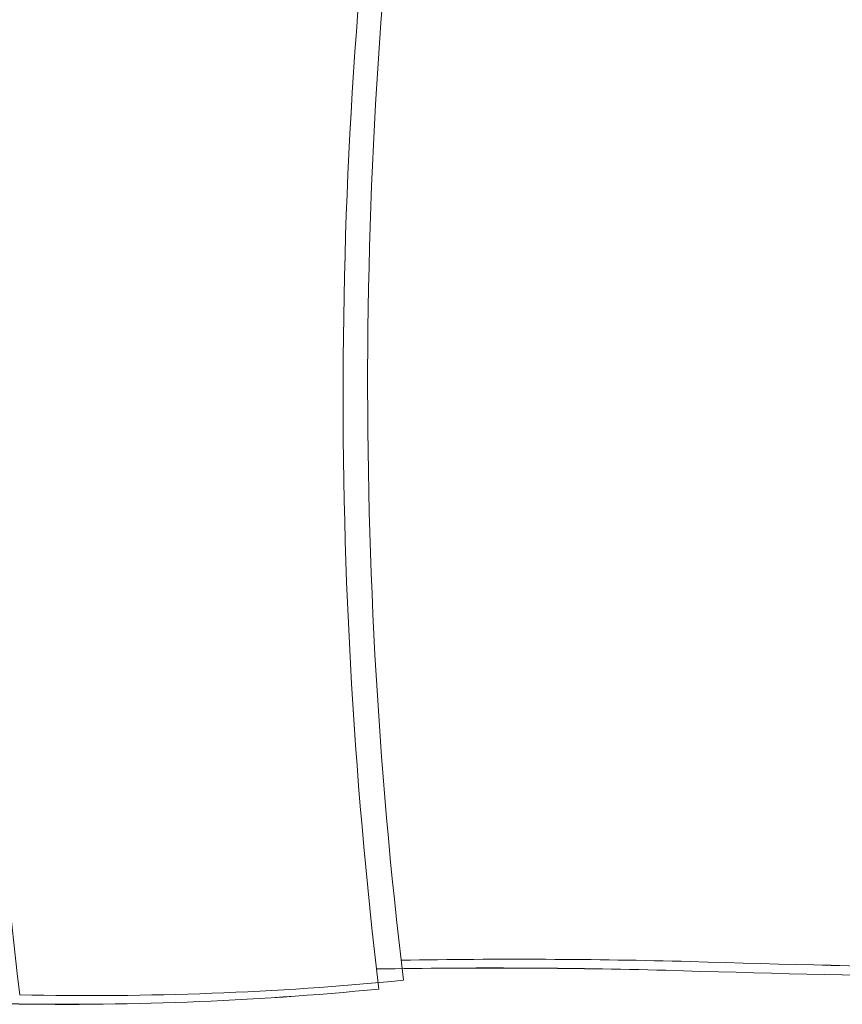
# Model space of a CAD drawing. Units: inches. Extents: x 963 to 2075, y 289 to 2657.
# Tile 38 of 98: x 1534 to 1555, y 1590 to 1615. Entities that reach past the tile are written whole.
import ezdxf

# ---------------------------------------------------------------- set-up
doc = ezdxf.new("R2010")
doc.units = ezdxf.units.IN
doc.layers.add('A-FURN', color=8, linetype='Continuous', lineweight=18)

# ---------------------------------------------------------------- blocks, each defined once
blk = doc.blocks.new('BED-DOUBLE')
for centre, radius, start, end in [((1234.775, 2369.061), 83.306, 88.72178, 95.60397), ((1234.775, 2369.062), 83.306, 88.72178, 95.60397), ((1234.136, 2368.833), 83.306, 88.72178, 95.60397), ((1234.136, 2368.833), 83.306, 88.72178, 95.60397), ((1072.18, 2432.636), 164.969, 356.08655, 6.78213), ((1097.916, 2436.239), 129.02, 351.78449, 6.90062), ((1097.916, 2436.239), 129.02, 351.78449, 6.90062), ((1098.555, 2436.467), 129.02, 351.78449, 6.90062), ((1098.555, 2436.468), 129.02, 351.78449, 6.90062), ((1203.619, 1969.172), 482.31, 88.22771, 91.71854), ((1203.619, 1969.173), 482.31, 88.22771, 91.71854), ((1204.258, 1969.401), 482.31, 88.22771, 91.71854), ((1204.258, 1969.401), 482.31, 88.22771, 91.71854), ((1223.698, 2621.53), 170.11, 268.4762, 271.00819), ((1223.698, 2621.531), 170.11, 268.4762, 271.00819), ((1223.059, 2621.302), 170.11, 268.4762, 271.00819), ((1223.059, 2621.302), 170.11, 268.4762, 271.00819)]:
    blk.add_arc(centre, radius, start, end)

msp = doc.modelspace()

# ---------------------------------------------------------------- block references
at = {"layer": 'A-FURN', "rotation": 180}
msp.add_blockref('BED-DOUBLE', (2769.937, 4041.99), dxfattribs=at)

doc.saveas('drawing.dxf')
